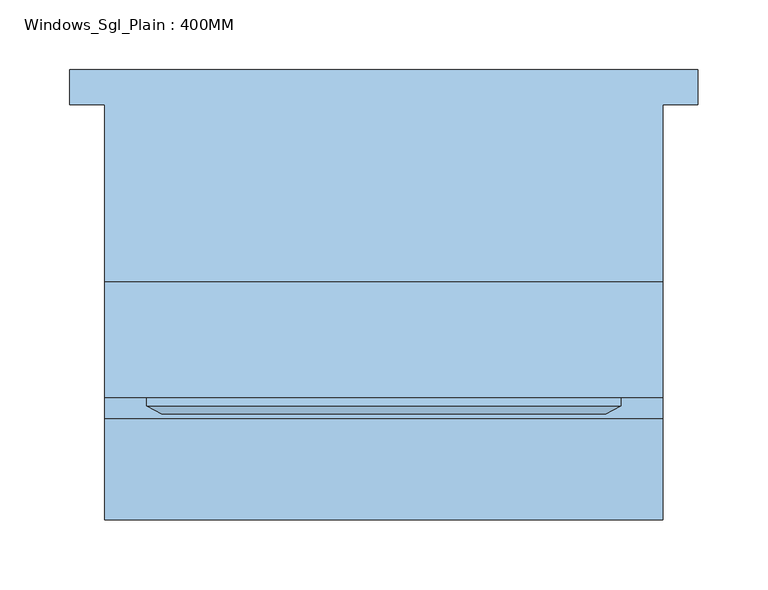
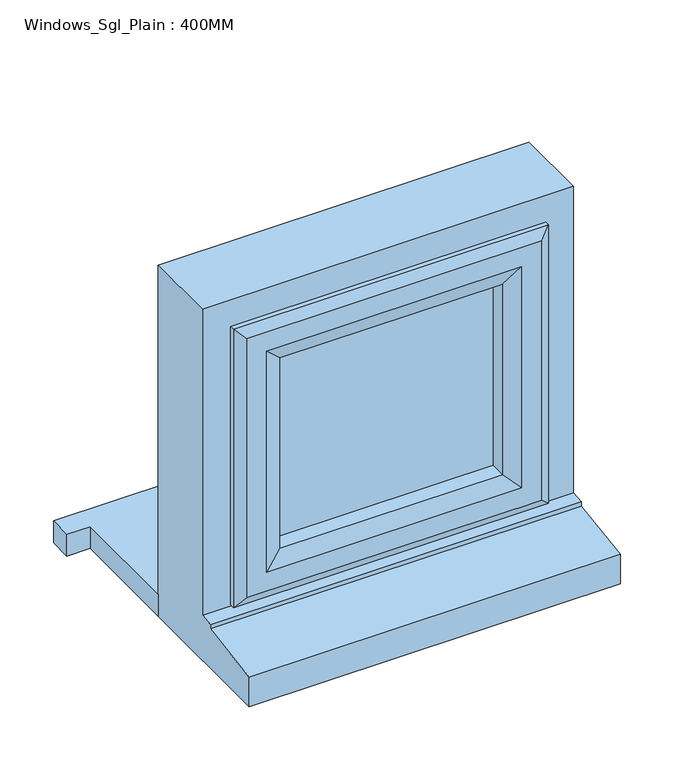
"""IFC4 building model written with IfcOpenShell, lengths in millimetres: window geometry, Windows_Sgl_Plain : 400MM."""

from ifc_helpers import new_model, si_unit, frame, origin, place, context, project, spatial, polyline, outline, extrude, faceted_brep, source, transform, mapped, element, save


def windows_sgl_plain_400mm_a5a4ca73(model_context):
    return source(origin(), model_context, "Body", "SolidModel", [
        extrude(outline(polyline([(-225.0, 146.5434322), (225.0, 146.5434322), (225.0, 121.5434322), (200.0, 121.5434322), (200.0, -5.4565678), (-200.0, -5.4565678), (-200.0, 121.5434322), (-225.0, 121.5434322), (-225.0, 146.5434322)])), frame((0.0, 0.0, 1710.0), z_axis=(0.0, 0.0, 1.0), x_axis=(1.0, 0.0, 0.0)), (0.0, 0.0, 1.0), 25.0),
        faceted_brep([(-200.0, -5.4565678, 1710.0), (-200.0, -5.4565678, 2110.0), (200.0, -5.4565678, 2110.0), (200.0, -5.4565678, 1710.0), (-140.0, -5.4565678, 2050.0), (-140.0, -5.4565678, 1785.0), (140.0, -5.4565678, 1785.0), (140.0, -5.4565678, 2050.0), (-200.0, -175.9565678, 1710.0), (-200.0, -175.9565678, 1743.8088847), (-200.0, -103.4565678, 1754.7449676), (-200.0, -103.4565678, 1759.68767), (-200.0, -88.4565678, 1761.0), (-200.0, -88.4565678, 2110.0), (200.0, -88.4565678, 1761.0), (200.0, -88.4565678, 2110.0), (-160.0, -88.4565678, 2070.0), (160.0, -88.4565678, 2070.0), (160.0, -88.4565678, 1773.0), (-160.0, -88.4565678, 1773.0), (-160.0, -23.4565678, 1773.0), (-160.0, -23.4565678, 2070.0), (160.0, -23.4565678, 1773.0), (160.0, -23.4565678, 2070.0), (-140.0, -23.4565678, 2050.0), (140.0, -23.4565678, 2050.0), (140.0, -23.4565678, 1785.0), (-140.0, -23.4565678, 1785.0), (200.0, -103.4565678, 1759.68767), (200.0, -103.4565678, 1754.7449676), (200.0, -175.9565678, 1743.8088847), (200.0, -175.9565678, 1710.0)], [[[0, 1, 2, 3], [4, 5, 6, 7]], [[0, 8, 9, 10, 11, 12, 13, 1]], [[12, 14, 15, 13], [16, 17, 18, 19]], [[19, 20, 21, 16]], [[21, 20, 22, 23], [24, 25, 26, 27]], [[24, 27, 5, 4]], [[1, 13, 15, 2]], [[16, 21, 23, 17]], [[7, 25, 24, 4]], [[14, 28, 29, 30, 31, 3, 2, 15]], [[17, 23, 22, 18]], [[7, 6, 26, 25]], [[31, 8, 0, 3]], [[30, 9, 8, 31]], [[29, 10, 9, 30]], [[28, 11, 10, 29]], [[14, 12, 11, 28]], [[20, 19, 18, 22]], [[5, 27, 26, 6]]]),
        extrude(outline(polyline([(130.0, -52.4565678), (130.0, -76.4565678), (-130.0, -76.4565678), (-130.0, -52.4565678), (130.0, -52.4565678)])), frame((0.0, 0.0, 1803.0), z_axis=(0.0, 0.0, 1.0), x_axis=(1.0, 0.0, 0.0)), (0.0, 0.0, 1.0), 237.0),
        faceted_brep([(-170.0, -88.4565678, 2080.0), (-170.0, -88.4565678, 1763.0), (-170.0, -94.2300705, 1763.0), (-170.0, -94.2300705, 2080.0), (-160.0, -23.4565678, 2070.0), (-160.0, -23.4565678, 1773.0), (-160.0, -88.4565678, 1773.0), (-160.0, -88.4565678, 2070.0), (-120.0, -37.9494677, 2030.0), (-120.0, -37.9494677, 1813.0), (-130.1480377, -23.4565678, 1802.8519623), (-130.1480377, -23.4565678, 2040.1480377), (-120.0, -52.4565678, 2030.0), (-120.0, -52.4565678, 1813.0), (-130.0, -76.4565678, 2040.0), (-130.0, -76.4565678, 1803.0), (-130.0, -52.4565678, 1803.0), (-130.0, -52.4565678, 2040.0), (-120.0, -94.2300705, 2030.0), (-120.0, -94.2300705, 1813.0), (-120.0, -76.4565678, 1813.0), (-120.0, -76.4565678, 2030.0), (-137.4457548, -100.0035732, 2047.4457548), (-137.4457548, -100.0035732, 1795.5542452), (-159.2153903, -100.0035732, 1773.7846097), (-159.2153903, -100.0035732, 2069.2153903), (170.0, -88.4565678, 1763.0), (170.0, -94.2300705, 1763.0), (160.0, -23.4565678, 1773.0), (160.0, -88.4565678, 1773.0), (120.0, -37.9494677, 1813.0), (130.1480377, -23.4565678, 1802.8519623), (120.0, -52.4565678, 1813.0), (130.0, -76.4565678, 1803.0), (130.0, -52.4565678, 1803.0), (120.0, -94.2300705, 1813.0), (120.0, -76.4565678, 1813.0), (137.4457548, -100.0035732, 1795.5542452), (159.2153903, -100.0035732, 1773.7846097), (170.0, -88.4565678, 2080.0), (170.0, -94.2300705, 2080.0), (160.0, -23.4565678, 2070.0), (160.0, -88.4565678, 2070.0), (120.0, -37.9494677, 2030.0), (130.1480377, -23.4565678, 2040.1480377), (120.0, -52.4565678, 2030.0), (130.0, -76.4565678, 2040.0), (130.0, -52.4565678, 2040.0), (120.0, -94.2300705, 2030.0), (120.0, -76.4565678, 2030.0), (137.4457548, -100.0035732, 2047.4457548), (159.2153903, -100.0035732, 2069.2153903)], [[[0, 1, 2, 3]], [[4, 5, 6, 7]], [[8, 9, 10, 11]], [[12, 13, 9, 8]], [[14, 15, 16, 17]], [[18, 19, 20, 21]], [[22, 23, 19, 18]], [[3, 2, 24, 25]], [[1, 26, 27, 2]], [[5, 28, 29, 6]], [[9, 30, 31, 10]], [[13, 32, 30, 9]], [[15, 33, 34, 16]], [[19, 35, 36, 20]], [[23, 37, 35, 19]], [[2, 27, 38, 24]], [[26, 39, 40, 27]], [[28, 41, 42, 29]], [[30, 43, 44, 31]], [[32, 45, 43, 30]], [[33, 46, 47, 34]], [[35, 48, 49, 36]], [[37, 50, 48, 35]], [[27, 40, 51, 38]], [[39, 0, 3, 40]], [[1, 0, 39, 26], [7, 6, 29, 42]], [[41, 4, 7, 42]], [[5, 4, 41, 28], [11, 10, 31, 44]], [[43, 8, 11, 44]], [[45, 12, 8, 43]], [[17, 16, 34, 47], [13, 12, 45, 32]], [[46, 14, 17, 47]], [[15, 14, 46, 33], [21, 20, 36, 49]], [[48, 18, 21, 49]], [[50, 22, 18, 48]], [[25, 24, 38, 51], [23, 22, 50, 37]], [[40, 3, 25, 51]]]),
    ])


if __name__ == "__main__":
    model = new_model("IFC4")
    model_context = context("Model", 3, world=origin())
    ifc_project = project(units=[si_unit("LENGTHUNIT", "METRE", prefix="MILLI")], contexts=[model_context])
    site = spatial("IfcSite", under=ifc_project)
    building = spatial("IfcBuilding", under=site)
    placement = place(None, origin())
    windows_sgl_plain_400mm_shape = windows_sgl_plain_400mm_a5a4ca73(model_context)
    element("IfcWindow", 1, ObjectType="Windows_Sgl_Plain : 400MM", at=placement, inside=building, context=model_context, shape_type="MappedRepresentation", body=[
        mapped(windows_sgl_plain_400mm_shape, transform((0.0, 0.0, 0.0), x_axis=(1.0, 0.0, 0.0), y_axis=(0.0, 1.0, 0.0), z_axis=(0.0, 0.0, 1.0))),
    ])
    save(model, "model.ifc")

# Revit data of these elements
# Type "Windows_Sgl_Plain : 400MM"
#   Type Mark = "65"
#   Operation = "SinglePanel"
#   Construction Type Id = "SGL"
#   Manufacturer = "Revit"
#   Keynote = "L10"
#   Analytic Construction = "Large single-glazed windows"
#   Wrap Layers (Ext) from Ext = 102.5 mm
#   Wrap Layers (Int) from Ext = 177.5 mm
#   Window Board Projection = 25 mm
#   Window Board Extension = 25 mm
#   Visual Light Transmittance = 0.9
#   Solar Heat Gain Coefficient = 0.86
#   Rough Width = 400 mm
#   Rough Height = 400 mm
#   Height = 400 mm
#   Width = 400 mm
#   Heat Transfer Coefficient (U) = 5.5617 W/(m²·K)
#   Glazing Thickness = 24 mm
#   FrameOffset - External = 50 mm
#   Frame Depth = 65 mm
#   Default Head Height = 2110 mm
#   Cill Depth = 87.5 mm
#   Cavity Closer Width = 50 mm
#   Cavity Closer Offset from Ext = 102.5 mm
#   Cavity Closer Depth = 85 mm
#   Vis - Cavity Closers = yes
#   Define Thermal Properties by = 1
#   Material Trim = Window Frame
#   Material Glass = Glass
#   Material Frame = Window Frame
#   Wall Closure = (empty or 0)
# Element 1 (IfcWindow, "Windows_Sgl_Plain : 400MM")
#   Materials on its faces: "Window Frame", "Glass"
# Materials
#   "Window Frame": colour RGB 249 249 249, transparency 0, Keynote = "L10", Cost = 0
#   "Glass": class "Glass", colour RGB 0 128 192, transparency 0.9, Description = "Soda Lime Glass", Cost = 0
